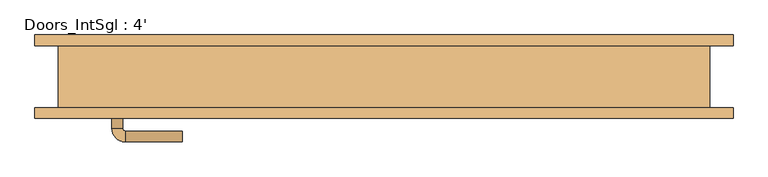
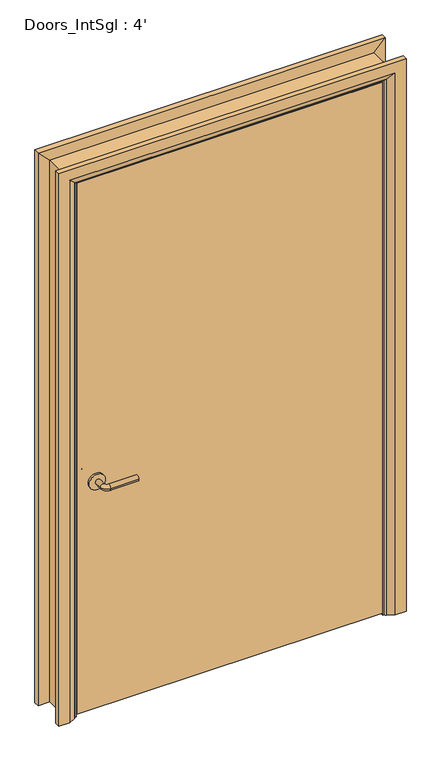
"""IFC4 building model written with IfcOpenShell, lengths in millimetres: door geometry, Doors_IntSgl : 4'."""

from ifc_helpers import new_model, si_unit, point, frame, frame_2d, origin, place, context, project, spatial, polyline, circle_curve, ellipse_curve, trimmed, segment, composite_curve, outline, extrude, faceted_brep, source, transform, mapped, element, save
from ifc_brep_helpers import plane_surface, cylinder_surface, revolved_surface, advanced_brep


def doors_intsgl_4_41b074ad(model_context):
    return source(origin(), model_context, "Body", "SolidModel", [
        advanced_brep(
        [(-502.6, -11.15, 900.0), (-482.6, -11.15, 900.0), (-502.6, 18.85, 900.0), (-482.6, 18.85, 900.0), (-477.6, 23.85, 900.0), (-477.6, 43.85, 900.0), (-372.6, 43.85, 900.0), (-372.6, 23.85, 900.0)],
        [
            (0, 1, circle_curve(frame((-492.6, -11.15, 900.0), z_axis=(0.0, -1.0, 0.0), x_axis=(1.0, 0.0, 0.0)), 10.0)),
            (1, 0, circle_curve(frame((-492.6, -11.15, 900.0), z_axis=(0.0, -1.0, 0.0), x_axis=(1.0, 0.0, 0.0)), 10.0)),
            (0, 2),
            (2, 3, circle_curve(frame((-492.6, 18.85, 900.0), z_axis=(0.0, -1.0, 0.0), x_axis=(1.0, 0.0, 0.0)), 10.0)),
            (3, 1),
            (3, 2, circle_curve(frame((-492.6, 18.85, 900.0), z_axis=(0.0, -1.0, 0.0), x_axis=(1.0, 0.0, 0.0)), 10.0)),
            (4, 3, circle_curve(frame((-477.6, 18.85, 900.0), z_axis=(0.0, 0.0, 1.0), x_axis=(-1.0, 0.0, 0.0)), 5.0)),
            (2, 5, circle_curve(frame((-477.6, 18.85, 900.0), z_axis=(0.0, 0.0, -1.0), x_axis=(-1.0, 0.0, 0.0)), 25.0)),
            (5, 4, circle_curve(frame((-477.6, 33.85, 900.0), z_axis=(-1.0, 0.0, 0.0), x_axis=(0.0, -1.0, 0.0)), 10.0)),
            (4, 5, circle_curve(frame((-477.6, 33.85, 900.0), z_axis=(-1.0, 0.0, 0.0), x_axis=(0.0, -1.0, 0.0)), 10.0)),
            (6, 7, circle_curve(frame((-372.6, 33.85, 900.0), z_axis=(1.0, 0.0, 0.0), x_axis=(0.0, -1.0, 0.0)), 10.0)),
            (7, 6, circle_curve(frame((-372.6, 33.85, 900.0), z_axis=(1.0, 0.0, 0.0), x_axis=(0.0, -1.0, 0.0)), 10.0)),
            (5, 6),
            (7, 4),
        ],
        [
            plane_surface(frame((-492.6, -11.15, 900.0), z_axis=(0.0, -1.0, 0.0), x_axis=(0.0, 0.0, 1.0))),
            cylinder_surface(frame((-492.6, -11.15, 900.0), z_axis=(0.0, -1.0, 0.0), x_axis=(1.0, 0.0, 0.0)), 10.0),
            revolved_surface(trimmed(ellipse_curve(frame((-492.6, 18.85, 900.0), z_axis=(0.0, -1.0, 0.0), x_axis=(1.0, 0.0, 0.0)), 10.0, 10.0), [point((-502.6, 18.85, 900.0))], [point((-482.6, 18.85, 900.0))], True, "CARTESIAN"), (-477.6, 18.85, 900.0), (0.0, 0.0, -1.0)),
            revolved_surface(trimmed(ellipse_curve(frame((-492.6, 18.85, 900.0), z_axis=(0.0, -1.0, 0.0), x_axis=(1.0, 0.0, 0.0)), 10.0, 10.0), [point((-482.6, 18.85, 900.0))], [point((-502.6, 18.85, 900.0))], True, "CARTESIAN"), (-477.6, 18.85, 900.0), (0.0, 0.0, -1.0)),
            plane_surface(frame((-372.6, 33.85, 900.0), z_axis=(1.0, 0.0, 0.0), x_axis=(0.0, 0.0, 1.0))),
            cylinder_surface(frame((-477.6, 33.85, 900.0), z_axis=(-1.0, 0.0, 0.0), x_axis=(0.0, -1.0, 0.0)), 10.0),
        ],
        [
            (0, [[1, 2]]),
            (1, [[-1, 3, 4, 5]]),
            (1, [[-2, -5, 6, -3]]),
            (2, [[7, -4, 8, 9]]),
            (3, [[-8, -6, -7, 10]]),
            (4, [[11, 12]]),
            (5, [[-9, 13, -12, 14]]),
            (5, [[-10, -14, -11, -13]]),
        ],
    ),
        extrude(outline(composite_curve([segment(trimmed(circle_curve(frame_2d((900.0, -495.1)), 30.0), [point((900.0, -525.1))], [point((900.0, -465.1))], False, "CARTESIAN"), True, "CONTINUOUS"), segment(trimmed(circle_curve(frame_2d((900.0, -495.1)), 30.0), [point((900.0, -465.1))], [point((900.0, -525.1))], False, "CARTESIAN"), True, "CONTINUOUS")], self_intersect=False)), frame((0.0, -19.15, 0.0), z_axis=(0.0, 1.0, 0.0), x_axis=(0.0, 0.0, 1.0)), (0.0, 0.0, 1.0), 8.0),
        advanced_brep(
        [(-502.6, -65.15, 900.0), (-482.6, -65.15, 900.0), (-482.6, -95.15, 900.0), (-502.6, -95.15, 900.0), (-477.6, -100.15, 900.0), (-477.6, -120.15, 900.0), (-372.6, -120.15, 900.0), (-372.6, -100.15, 900.0)],
        [
            (0, 1, circle_curve(frame((-492.6, -65.15, 900.0), z_axis=(0.0, 1.0, 0.0), x_axis=(1.0, 0.0, 0.0)), 10.0)),
            (1, 0, circle_curve(frame((-492.6, -65.15, 900.0), z_axis=(0.0, 1.0, 0.0), x_axis=(1.0, 0.0, 0.0)), 10.0)),
            (1, 2),
            (2, 3, circle_curve(frame((-492.6, -95.15, 900.0), z_axis=(0.0, 1.0, 0.0), x_axis=(1.0, 0.0, 0.0)), 10.0)),
            (3, 0),
            (3, 2, circle_curve(frame((-492.6, -95.15, 900.0), z_axis=(0.0, 1.0, 0.0), x_axis=(1.0, 0.0, 0.0)), 10.0)),
            (4, 5, circle_curve(frame((-477.6, -110.15, 900.0), z_axis=(-1.0, 0.0, 0.0), x_axis=(0.0, 1.0, 0.0)), 10.0)),
            (5, 3, circle_curve(frame((-477.6, -95.15, 900.0), z_axis=(0.0, 0.0, -1.0), x_axis=(-1.0, 0.0, 0.0)), 25.0)),
            (2, 4, circle_curve(frame((-477.6, -95.15, 900.0), z_axis=(0.0, 0.0, 1.0), x_axis=(-1.0, 0.0, 0.0)), 5.0)),
            (5, 4, circle_curve(frame((-477.6, -110.15, 900.0), z_axis=(-1.0, 0.0, 0.0), x_axis=(0.0, 1.0, 0.0)), 10.0)),
            (6, 7, circle_curve(frame((-372.6, -110.15, 900.0), z_axis=(1.0, 0.0, 0.0), x_axis=(0.0, 1.0, 0.0)), 10.0)),
            (7, 6, circle_curve(frame((-372.6, -110.15, 900.0), z_axis=(1.0, 0.0, 0.0), x_axis=(0.0, 1.0, 0.0)), 10.0)),
            (4, 7),
            (6, 5),
        ],
        [
            plane_surface(frame((-492.6, -65.15, 900.0), z_axis=(0.0, 1.0, 0.0), x_axis=(0.0, 0.0, 1.0))),
            cylinder_surface(frame((-492.6, -65.15, 900.0), z_axis=(0.0, 1.0, 0.0), x_axis=(1.0, 0.0, 0.0)), 10.0),
            revolved_surface(trimmed(ellipse_curve(frame((-492.6, -95.15, 900.0), z_axis=(0.0, -1.0, 0.0), x_axis=(1.0, 0.0, 0.0)), 10.0, 10.0), [point((-502.6, -95.15, 900.0))], [point((-482.6, -95.15, 900.0))], True, "CARTESIAN"), (-477.6, -95.15, 900.0), (0.0, 0.0, -1.0)),
            revolved_surface(trimmed(ellipse_curve(frame((-492.6, -95.15, 900.0), z_axis=(0.0, -1.0, 0.0), x_axis=(1.0, 0.0, 0.0)), 10.0, 10.0), [point((-482.6, -95.15, 900.0))], [point((-502.6, -95.15, 900.0))], True, "CARTESIAN"), (-477.6, -95.15, 900.0), (0.0, 0.0, -1.0)),
            plane_surface(frame((-372.6, -110.15, 900.0), z_axis=(1.0, 0.0, 0.0), x_axis=(0.0, 0.0, 1.0))),
            cylinder_surface(frame((-477.6, -110.15, 900.0), z_axis=(-1.0, 0.0, 0.0), x_axis=(0.0, 1.0, 0.0)), 10.0),
        ],
        [
            (0, [[1, 2]]),
            (1, [[3, 4, 5, -2]]),
            (1, [[-5, 6, -3, -1]]),
            (2, [[7, 8, -4, 9]]),
            (3, [[10, -9, -6, -8]]),
            (4, [[11, 12]]),
            (5, [[13, -11, 14, -7]]),
            (5, [[-14, -12, -13, -10]]),
        ],
    ),
        extrude(outline(composite_curve([segment(trimmed(circle_curve(frame_2d((900.0, -495.1)), 30.0), [point((900.0, -525.1))], [point((900.0, -465.1))], False, "CARTESIAN"), True, "CONTINUOUS"), segment(trimmed(circle_curve(frame_2d((900.0, -495.1)), 30.0), [point((900.0, -465.1))], [point((900.0, -525.1))], False, "CARTESIAN"), True, "CONTINUOUS")], self_intersect=False)), frame((0.0, -65.15, 0.0), z_axis=(0.0, 1.0, 0.0), x_axis=(0.0, 0.0, 1.0)), (0.0, 0.0, 1.0), 8.0),
        extrude(outline(polyline([(567.6, -19.15), (567.6, -57.15), (-567.6, -57.15), (-567.6, -19.15), (567.6, -19.15)])), frame((0.0, 0.0, 8.0), z_axis=(0.0, 0.0, 1.0), x_axis=(1.0, 0.0, 0.0)), (0.0, 0.0, 1.0), 2083.6),
        advanced_brep(
        [(644.6, -77.15, 0.0), (604.6, -77.15, 0.0), (578.6, -63.15, 0.0), (574.6, -57.15, 0.0), (644.6, -57.15, 0.0), (644.6, -57.15, 2168.6), (644.6, -77.15, 2168.6), (574.6, -57.15, 2098.6), (-574.6, -57.15, 2098.6), (-574.6, -57.15, 0.0), (-644.6, -57.15, 0.0), (-644.6, -57.15, 2168.6), (578.6, -63.15, 2102.6), (604.6, -77.15, 2128.6), (-644.6, -77.15, 2168.6), (-644.6, -77.15, 0.0), (-604.6, -77.15, 0.0), (-604.6, -77.15, 2128.6), (-578.6, -63.15, 0.0), (-578.6, -63.15, 2102.6)],
        [
            (0, 1),
            (1, 2),
            (2, 3, circle_curve(frame((582.6, -56.15, 0.0), z_axis=(0.0, 0.0, -1.0), x_axis=(1.0, 0.0, 0.0)), 8.0622577)),
            (3, 4),
            (4, 0),
            (4, 5),
            (5, 6),
            (6, 0),
            (3, 7),
            (7, 8),
            (8, 9),
            (9, 10),
            (10, 11),
            (11, 5),
            (2, 12),
            (12, 7, ellipse_curve(frame((582.6, -56.15, 2106.6), z_axis=(0.7071067811865475, 0.0, -0.7071067811865475), x_axis=(-0.7071067811865474, 0.0, -0.7071067811865476)), 11.4017543, 8.0622577)),
            (1, 13),
            (13, 12),
            (6, 14),
            (14, 15),
            (15, 16),
            (16, 17),
            (17, 13),
            (10, 15),
            (14, 11),
            (9, 18, circle_curve(frame((-582.6, -56.15, 0.0), z_axis=(0.0, 0.0, -1.0), x_axis=(-1.0, 0.0, 0.0)), 8.0622577)),
            (18, 16),
            (19, 18),
            (8, 19, ellipse_curve(frame((-582.6, -56.15, 2106.6), z_axis=(-0.7071067811865475, 0.0, -0.7071067811865475), x_axis=(-0.7071067811865474, 0.0, 0.7071067811865476)), 11.4017543, 8.0622577)),
            (19, 17),
            (12, 19),
        ],
        [
            plane_surface(frame((574.6, -57.15, 0.0), z_axis=(0.0, 0.0, -1.0), x_axis=(0.0, 1.0, 0.0))),
            plane_surface(frame((644.6, -77.15, 0.0), z_axis=(1.0, 0.0, 0.0), x_axis=(0.0, 0.0, 1.0))),
            plane_surface(frame((644.6, -57.15, 0.0), z_axis=(0.0, 1.0, 0.0), x_axis=(0.0, 0.0, 1.0))),
            cylinder_surface(frame((582.6, -56.15, 0.0), z_axis=(0.0, 0.0, -1.0), x_axis=(1.0, 0.0, 0.0)), 8.0622577),
            plane_surface(frame((578.6, -63.15, 0.0), z_axis=(-0.4740998230350126, -0.880471099922178, 0.0), x_axis=(0.0, 0.0, 1.0))),
            plane_surface(frame((604.6, -77.15, 0.0), z_axis=(0.0, -1.0, 0.0), x_axis=(0.0, 0.0, 1.0))),
            plane_surface(frame((-644.6, -77.15, 2168.6), z_axis=(-1.0, 0.0, 0.0), x_axis=(0.0, 0.0, -1.0))),
            plane_surface(frame((-574.6, -57.15, 0.0), z_axis=(0.0, 0.0, -1.0), x_axis=(0.0, 1.0, 0.0))),
            cylinder_surface(frame((-582.6, -56.15, 2098.6), z_axis=(0.0, 0.0, 1.0), x_axis=(-1.0, 0.0, 0.0)), 8.0622577),
            plane_surface(frame((-578.6, -63.15, 2102.6), z_axis=(0.47409982303501824, -0.8804710999221749, 0.0), x_axis=(0.0, 0.0, -1.0))),
            plane_surface(frame((644.6, -77.15, 2168.6), z_axis=(0.0, 0.0, 1.0), x_axis=(-1.0, 0.0, 0.0))),
            cylinder_surface(frame((574.6, -56.15, 2106.6), z_axis=(1.0, 0.0, 0.0), x_axis=(0.0, 0.0, 1.0)), 8.0622577),
            plane_surface(frame((578.6, -63.15, 2102.6), z_axis=(0.0, -0.8804710999221764, -0.4740998230350154), x_axis=(-1.0, 0.0, 0.0))),
        ],
        [
            (0, [[1, 2, 3, 4, 5]]),
            (1, [[6, 7, 8, -5]]),
            (2, [[9, 10, 11, 12, 13, 14, -6, -4]]),
            (3, [[15, 16, -9, -3]]),
            (4, [[17, 18, -15, -2]]),
            (5, [[-8, 19, 20, 21, 22, 23, -17, -1]]),
            (6, [[-13, 24, -20, 25]]),
            (7, [[-24, -12, 26, 27, -21]]),
            (8, [[28, -26, -11, 29]]),
            (9, [[-22, -27, -28, 30]]),
            (10, [[-14, -25, -19, -7]]),
            (11, [[31, -29, -10, -16]]),
            (12, [[-23, -30, -31, -18]]),
        ],
    ),
        extrude(outline(polyline([(0.0, -550.6), (2074.6, -550.6), (2074.6, 550.6), (0.0, 550.6), (0.0, 569.6), (2093.6, 569.6), (2093.6, -569.6), (0.0, -569.6), (0.0, -550.6)])), frame((0.0, -17.15, 0.0), z_axis=(0.0, 1.0, 0.0), x_axis=(0.0, 0.0, 1.0)), (0.0, 0.0, 1.0), 32.0),
        advanced_brep(
        [(-644.6, 77.15, 0.0), (-604.6, 77.15, 0.0), (-578.6, 63.15, 0.0), (-574.6, 57.15, 0.0), (-644.6, 57.15, 0.0), (-644.6, 57.15, 2168.6), (-644.6, 77.15, 2168.6), (-574.6, 57.15, 2098.6), (-578.6, 63.15, 2102.6), (-604.6, 77.15, 2128.6), (644.6, 77.15, 0.0), (644.6, 57.15, 0.0), (574.6, 57.15, 0.0), (578.6, 63.15, 0.0), (604.6, 77.15, 0.0), (644.6, 77.15, 2168.6), (604.6, 77.15, 2128.6), (578.6, 63.15, 2102.6), (574.6, 57.15, 2098.6), (644.6, 57.15, 2168.6)],
        [
            (0, 1),
            (1, 2),
            (2, 3, circle_curve(frame((-582.6, 56.15, 0.0), z_axis=(0.0, 0.0, -1.0), x_axis=(-1.0, 0.0, 0.0)), 8.0622577)),
            (3, 4),
            (4, 0),
            (4, 5),
            (5, 6),
            (6, 0),
            (3, 7),
            (7, 5),
            (2, 8),
            (8, 7, ellipse_curve(frame((-582.6, 56.15, 2106.6), z_axis=(-0.7071067811865475, 0.0, -0.7071067811865475), x_axis=(0.7071067811865474, 0.0, -0.7071067811865476)), 11.4017543, 8.0622577)),
            (1, 9),
            (9, 8),
            (6, 9),
            (10, 11),
            (11, 12),
            (12, 13, circle_curve(frame((582.6, 56.15, 0.0), z_axis=(0.0, 0.0, -1.0), x_axis=(1.0, 0.0, 0.0)), 8.0622577)),
            (13, 14),
            (14, 10),
            (15, 10),
            (14, 16),
            (16, 15),
            (13, 17),
            (17, 16),
            (12, 18),
            (18, 17, ellipse_curve(frame((582.6, 56.15, 2106.6), z_axis=(0.7071067811865475, 0.0, -0.7071067811865475), x_axis=(0.7071067811865474, 0.0, 0.7071067811865476)), 11.4017543, 8.0622577)),
            (11, 19),
            (19, 18),
            (15, 19),
            (5, 19),
            (15, 6),
            (7, 18),
            (8, 17),
            (9, 16),
        ],
        [
            plane_surface(frame((-574.6, 129.9510989, 0.0), z_axis=(0.0, 0.0, -1.0), x_axis=(1.0, 0.0, 0.0))),
            plane_surface(frame((-644.6, 77.15, 0.0), z_axis=(-1.0, 0.0, 0.0), x_axis=(0.0, 0.0, 1.0))),
            plane_surface(frame((-644.6, 57.15, 0.0), z_axis=(0.0, -1.0, 0.0), x_axis=(0.0, 0.0, 1.0))),
            cylinder_surface(frame((-582.6, 56.15, 0.0), z_axis=(0.0, 0.0, -1.0), x_axis=(-1.0, 0.0, 0.0)), 8.0622577),
            plane_surface(frame((-578.6, 63.15, 0.0), z_axis=(0.4740998230350183, 0.8804710999221749, 0.0), x_axis=(0.0, 0.0, 1.0))),
            plane_surface(frame((-604.6, 77.15, 0.0), z_axis=(0.0, 1.0, 0.0), x_axis=(0.0, 0.0, 1.0))),
            plane_surface(frame((574.6, 129.9510989, 0.0), z_axis=(0.0, 0.0, -1.0), x_axis=(-1.0, 0.0, 0.0))),
            plane_surface(frame((604.6, 77.15, 2128.6), z_axis=(0.0, 1.0, 0.0), x_axis=(0.0, 0.0, -1.0))),
            plane_surface(frame((578.6, 63.15, 2102.6), z_axis=(-0.4740998230350183, 0.8804710999221749, 0.0), x_axis=(0.0, 0.0, -1.0))),
            cylinder_surface(frame((582.6, 56.15, 2098.6), z_axis=(0.0, 0.0, 1.0), x_axis=(1.0, 0.0, 0.0)), 8.0622577),
            plane_surface(frame((644.6, 57.15, 2168.6), z_axis=(0.0, -1.0, 0.0), x_axis=(0.0, 0.0, -1.0))),
            plane_surface(frame((644.6, 77.15, 2168.6), z_axis=(1.0, 0.0, 0.0), x_axis=(0.0, 0.0, -1.0))),
            plane_surface(frame((-644.6, 77.15, 2168.6), z_axis=(0.0, 0.0, 1.0), x_axis=(1.0, 0.0, 0.0))),
            plane_surface(frame((-644.6, 57.15, 2168.6), z_axis=(0.0, -1.0, 0.0), x_axis=(1.0, 0.0, 0.0))),
            cylinder_surface(frame((-574.6, 56.15, 2106.6), z_axis=(-1.0, 0.0, 0.0), x_axis=(0.0, 0.0, 1.0)), 8.0622577),
            plane_surface(frame((-578.6, 63.15, 2102.6), z_axis=(0.0, 0.8804710999221749, -0.4740998230350183), x_axis=(1.0, 0.0, 0.0))),
            plane_surface(frame((-604.6, 77.15, 2128.6), z_axis=(0.0, 1.0, 0.0), x_axis=(1.0, 0.0, 0.0))),
        ],
        [
            (0, [[1, 2, 3, 4, 5]]),
            (1, [[6, 7, 8, -5]]),
            (2, [[9, 10, -6, -4]]),
            (3, [[11, 12, -9, -3]]),
            (4, [[13, 14, -11, -2]]),
            (5, [[-8, 15, -13, -1]]),
            (6, [[16, 17, 18, 19, 20]]),
            (7, [[21, -20, 22, 23]]),
            (8, [[-22, -19, 24, 25]]),
            (9, [[-24, -18, 26, 27]]),
            (10, [[-26, -17, 28, 29]]),
            (11, [[-28, -16, -21, 30]]),
            (12, [[31, -30, 32, -7]]),
            (13, [[33, -29, -31, -10]]),
            (14, [[34, -27, -33, -12]]),
            (15, [[35, -25, -34, -14]]),
            (16, [[-32, -23, -35, -15]]),
        ],
    ),
        faceted_brep([(-569.6, -57.15, 0.0), (-601.6, -57.15, 0.0), (-601.6, 57.15, 0.0), (-569.6, 57.15, 0.0), (-569.6, 57.15, 2093.6), (-569.6, -57.15, 2093.6), (-601.6, 57.15, 2125.6), (-601.6, -57.15, 2125.6), (569.6, -57.15, 0.0), (569.6, 57.15, 0.0), (601.6, 57.15, 0.0), (601.6, -57.15, 0.0), (569.6, -57.15, 2093.6), (601.6, -57.15, 2125.6), (601.6, 57.15, 2125.6), (569.6, 57.15, 2093.6)], [[[0, 1, 2, 3]], [[3, 4, 5, 0]], [[2, 6, 4, 3]], [[1, 7, 6, 2]], [[0, 5, 7, 1]], [[8, 9, 10, 11]], [[12, 8, 11, 13]], [[13, 11, 10, 14]], [[14, 10, 9, 15]], [[15, 9, 8, 12]], [[4, 15, 12, 5]], [[6, 14, 15, 4]], [[7, 13, 14, 6]], [[5, 12, 13, 7]]]),
    ])


if __name__ == "__main__":
    model = new_model("IFC4")
    model_context = context("Model", 3, world=origin())
    ifc_project = project(units=[si_unit("LENGTHUNIT", "METRE", prefix="MILLI")], contexts=[model_context])
    site = spatial("IfcSite", under=ifc_project)
    building = spatial("IfcBuilding", under=site)
    placement = place(None, origin())
    doors_intsgl_4_shape = doors_intsgl_4_41b074ad(model_context)
    element("IfcDoor", 1, ObjectType="Doors_IntSgl : 4'", at=placement, inside=building, context=model_context, shape_type="MappedRepresentation", body=[
        mapped(doors_intsgl_4_shape, transform((0.0, 0.0, 0.0), x_axis=(1.0, 0.0, 0.0), y_axis=(0.0, 1.0, 0.0), z_axis=(0.0, 0.0, 1.0))),
    ])
    save(model, "model.ifc")

# Revit data of these elements
# Type "Doors_IntSgl : 4'"
#   Type Mark = "49"
#   Type Comments = "Internal Single"
#   Operation = "SingleSwingRight"
#   Manufacturer = "Revit"
#   Keynote = "L20"
#   Description = "Internal Single Door"
#   Analytic Construction = "Metal"
#   UnderCut = 0' - 0.31496"
#   Tolerance = 0' - 0.07874"
#   Thickness = 0' - 1.49606"
#   Thermal Resistance (R) = 0.270117 (m²·K)/W
#   Structural Tolerance = 0' - 0.31496"
#   StopDepth = 0' - 1.25984"
#   Stop Thickness = 0' - 0.74803"
#   Rough Width = 4' - 0"
#   Rough Height = 7' - 0"
#   Height to Top Lock Rail = 3' - 3.37008"
#   Heat Transfer Coefficient (U) = 3.7021 W/(m²·K)
#   Handle Z Distance = 2' - 11.43307"
#   Handle X Distance = 0' - 2.95276"
#   Frame Thickness = 0' - 1.25984"
#   Door Panel Width = 3' - 8.69291"
#   Door Panel Thickness = 0' - 1.49606"
#   Door Panel Offset = 0' - 0"
#   Height = 7' - 0"
#   Width = 4' - 0"
#   Door Panel Height = 6' - 10.0315"
#   Architrave Setback = 0' - 0.19685"
#   Vis - Ironmongery = yes
#   Material Ironmongery = Door - Handle
#   Material Frame = Door - Frame/Mullion (1)
#   Material Door = Door - Panel
#   Material Architrave = Door - Architrave
#   Visual Light Transmittance = 0
#   Solar Heat Gain Coefficient = 0
#   Function = (empty or 0)
#   Wall Closure = (empty or 0)
# Element 1 (IfcDoor, "Doors_IntSgl : 4'")
#   Materials on its faces: "Door - Architrave", "Door - Handle", "Door - Frame/Mullion (1)", "Door - Panel"
# Materials
#   "Door - Handle": colour RGB 0 0 0, transparency 0, Keynote = "P21", Cost = 0
#   "Door - Frame/Mullion (1)": class "Wood", colour RGB 212 179 113, transparency 0, Keynote = "L20", Cost = 0
#   "Door - Panel": class "Wood", colour RGB 210 159 95, transparency 0, Keynote = "L20", Cost = 0
#   "Door - Architrave": class "Wood", colour RGB 154 90 5, transparency 0, Keynote = "P20", Cost = 0
